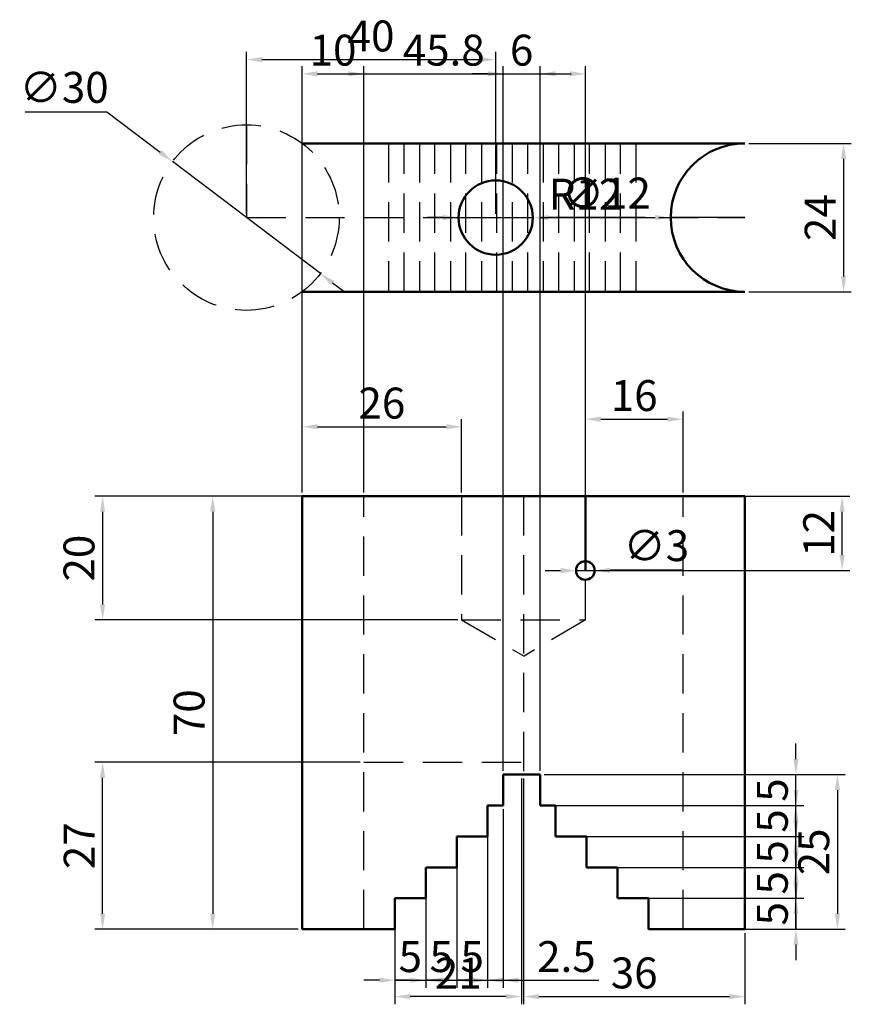
# Model space of a CAD drawing. Units: millimetres. Extents: x 1338 to 1892, y 1867 to 2306.
# Tile 1 of 3: x 1338 to 1473, y 1867 to 2026. Entities that reach past the tile are written whole.
import ezdxf

# ---------------------------------------------------------------- set-up
doc = ezdxf.new("R2010")
doc.units = ezdxf.units.MM
doc.linetypes.add('HIDDEN', pattern=[9.525, 6.35, -3.175])
for name, color, linetype, lineweight in [('M-DIMS', 2, 'Continuous', 25), ('M-HIDN', 4, 'HIDDEN', 25), ('M-OUTL', 7, 'Continuous', 50)]:
    doc.layers.add(name, color=color, linetype=linetype, lineweight=lineweight)
doc.styles.get("Standard").update_dxf_attribs({"font": 'arial.ttf'})
doc.dimstyles.new('ISO-25', dxfattribs={"dimtxt": 5, "dimasz": 2.5, "dimexe": 1.25, "dimexo": 0.625, "dimtad": 1, "dimtoh": 1, "dimdec": 0, "dimtxsty": 'Standard', "dimcen": 2.5, "dimadec": 0, "dimazin": 0, "dimtfac": 1, "dimtdec": 0, "dimtmove": 0, "dimatfit": 3, "dimfxl": 1, "dimarcsym": 0})

# ---------------------------------------------------------------- blocks, each defined once
blk = doc.blocks.new('*D16')
at = {"layer": 'Defpoints', "color": 0, "transparency": 16777216}
for p in [(1362.75, 2003.52), (1386.66, 1985.39)]:
    blk.add_point(p, dxfattribs=at)
at = {"layer": 'M-DIMS', "color": 0, "lineweight": -2, "transparency": 16777216}
for p, q in [((1338.95, 2011.54), (1352.16, 2011.54)), ((1352.16, 2011.54), (1360.76, 2005.03)), ((1386.66, 1985.39), (1362.75, 2003.52)), ((1388.65, 1983.88), (1390.65, 1982.37))]:
    blk.add_line(p, q, dxfattribs=at)
at = {"layer": 'M-DIMS', "color": 0, "transparency": 16777216}
for points in [[(1361.01, 2005.36), (1360.51, 2004.69), (1362.75, 2003.52)], [(1388.91, 1984.22), (1388.4, 1983.55), (1386.66, 1985.39)]]:
    blk.add_solid(points, dxfattribs=at)
at = {"layer": 'M-DIMS', "color": 0, "transparency": 16777216, "insert": (1345.24, 2014.86), "char_height": 5, "attachment_point": 5}
blk.add_mtext('∅30', dxfattribs=at)
blk = doc.blocks.new('*D17')
at = {"layer": 'Defpoints', "color": 0, "transparency": 16777216}
for p in [(1415.01, 2019.99), (1374.71, 1994.45), (1415.01, 1994.45)]:
    blk.add_point(p, dxfattribs=at)
at = {"layer": 'M-DIMS', "color": 0, "lineweight": -2, "transparency": 16777216}
for p, q in [((1374.71, 1995.08), (1374.71, 2021.24)), ((1415.01, 1995.08), (1415.01, 2021.24)), ((1377.21, 2019.99), (1412.51, 2019.99))]:
    blk.add_line(p, q, dxfattribs=at)
at = {"layer": 'M-DIMS', "color": 0, "transparency": 16777216}
for points in [[(1377.21, 2020.41), (1377.21, 2019.58), (1374.71, 2019.99)], [(1412.51, 2020.41), (1412.51, 2019.58), (1415.01, 2019.99)]]:
    blk.add_solid(points, dxfattribs=at)
at = {"layer": 'M-DIMS', "color": 0, "transparency": 16777216, "insert": (1394.86, 2023.17), "char_height": 5, "attachment_point": 5}
blk.add_mtext('40', dxfattribs=at)
blk = doc.blocks.new('*D18')
at = {"layer": 'Defpoints', "color": 0, "transparency": 16777216}
for p in [(1455.31, 2006.45), (1455.31, 1982.45), (1471.26, 1982.45)]:
    blk.add_point(p, dxfattribs=at)
at = {"layer": 'M-DIMS', "color": 0, "lineweight": -2, "transparency": 16777216}
for p, q in [((1455.93, 2006.45), (1472.51, 2006.45)), ((1471.26, 2003.95), (1471.26, 1984.95)), ((1455.93, 1982.45), (1472.51, 1982.45))]:
    blk.add_line(p, q, dxfattribs=at)
at = {"layer": 'M-DIMS', "color": 0, "transparency": 16777216}
for points in [[(1470.84, 2003.95), (1471.68, 2003.95), (1471.26, 2006.45)], [(1470.84, 1984.95), (1471.68, 1984.95), (1471.26, 1982.45)]]:
    blk.add_solid(points, dxfattribs=at)
at = {"layer": 'M-DIMS', "color": 0, "transparency": 16777216, "insert": (1468.13, 1994.45), "char_height": 5, "attachment_point": 5, "rotation": 90}
blk.add_mtext('24', dxfattribs=at)
blk = doc.blocks.new('*D19')
at = {"layer": 'Defpoints', "color": 0, "transparency": 16777216}
for p in [(1383.71, 1949.39), (1369.26, 1879.39), (1383.71, 1879.39)]:
    blk.add_point(p, dxfattribs=at)
at = {"layer": 'M-DIMS', "color": 0, "lineweight": -2, "transparency": 16777216}
for p, q in [((1383.08, 1949.39), (1368.01, 1949.39)), ((1369.26, 1946.89), (1369.26, 1881.89)), ((1383.08, 1879.39), (1368.01, 1879.39))]:
    blk.add_line(p, q, dxfattribs=at)
at = {"layer": 'M-DIMS', "color": 0, "transparency": 16777216}
for points in [[(1368.84, 1946.89), (1369.68, 1946.89), (1369.26, 1949.39)], [(1368.84, 1881.89), (1369.68, 1881.89), (1369.26, 1879.39)]]:
    blk.add_solid(points, dxfattribs=at)
at = {"layer": 'M-DIMS', "color": 0, "transparency": 16777216, "insert": (1366.08, 1914.39), "char_height": 5, "attachment_point": 5, "rotation": 90}
blk.add_mtext('70', dxfattribs=at)
blk = doc.blocks.new('*D20')
at = {"layer": 'Defpoints', "color": 0, "transparency": 16777216}
for p in [(1419.21, 1904.39), (1398.71, 1879.39), (1398.71, 1868.49)]:
    blk.add_point(p, dxfattribs=at)
at = {"layer": 'M-DIMS', "color": 0, "lineweight": -2, "transparency": 16777216}
for p, q in [((1419.21, 1903.77), (1419.21, 1867.24)), ((1398.71, 1878.77), (1398.71, 1867.24)), ((1416.71, 1868.49), (1401.21, 1868.49))]:
    blk.add_line(p, q, dxfattribs=at)
at = {"layer": 'M-DIMS', "color": 0, "transparency": 16777216}
for points in [[(1401.21, 1868.91), (1401.21, 1868.08), (1398.71, 1868.49)], [(1416.71, 1868.91), (1416.71, 1868.08), (1419.21, 1868.49)]]:
    blk.add_solid(points, dxfattribs=at)
at = {"layer": 'M-DIMS', "color": 0, "transparency": 16777216, "insert": (1408.96, 1871.63), "char_height": 5, "attachment_point": 5}
blk.add_mtext('21', dxfattribs=at)
blk = doc.blocks.new('*D21')
at = {"layer": 'Defpoints', "color": 0, "transparency": 16777216}
for p in [(1419.51, 1904.39), (1455.31, 1879.39), (1455.31, 1868.49)]:
    blk.add_point(p, dxfattribs=at)
at = {"layer": 'M-DIMS', "color": 0, "lineweight": -2, "transparency": 16777216}
for p, q in [((1419.51, 1903.77), (1419.51, 1867.24)), ((1455.31, 1878.77), (1455.31, 1867.24)), ((1422.01, 1868.49), (1452.81, 1868.49))]:
    blk.add_line(p, q, dxfattribs=at)
at = {"layer": 'M-DIMS', "color": 0, "transparency": 16777216}
for points in [[(1422.01, 1868.91), (1422.01, 1868.08), (1419.51, 1868.49)], [(1452.81, 1868.91), (1452.81, 1868.08), (1455.31, 1868.49)]]:
    blk.add_solid(points, dxfattribs=at)
at = {"layer": 'M-DIMS', "color": 0, "transparency": 16777216, "insert": (1437.41, 1871.67), "char_height": 5, "attachment_point": 5}
blk.add_mtext('36', dxfattribs=at)
blk = doc.blocks.new('*D22')
at = {"layer": 'Defpoints', "color": 0, "transparency": 16777216}
for p in [(1422.21, 1904.39), (1455.31, 1879.39), (1470.27, 1879.39)]:
    blk.add_point(p, dxfattribs=at)
at = {"layer": 'M-DIMS', "color": 0, "lineweight": -2, "transparency": 16777216}
for p, q in [((1422.83, 1904.39), (1471.52, 1904.39)), ((1470.27, 1901.89), (1470.27, 1881.89)), ((1455.93, 1879.39), (1471.52, 1879.39))]:
    blk.add_line(p, q, dxfattribs=at)
at = {"layer": 'M-DIMS', "color": 0, "transparency": 16777216}
for points in [[(1469.85, 1901.89), (1470.69, 1901.89), (1470.27, 1904.39)], [(1469.85, 1881.89), (1470.69, 1881.89), (1470.27, 1879.39)]]:
    blk.add_solid(points, dxfattribs=at)
at = {"layer": 'M-DIMS', "color": 0, "transparency": 16777216, "insert": (1467.09, 1891.89), "char_height": 5, "attachment_point": 5, "rotation": 90}
blk.add_mtext('25', dxfattribs=at)
blk = doc.blocks.new('*D23')
at = {"layer": 'Defpoints', "color": 0, "transparency": 16777216}
for p in [(1445.31, 1961.86), (1429.51, 1949.39), (1445.31, 1949.39)]:
    blk.add_point(p, dxfattribs=at)
at = {"layer": 'M-DIMS', "color": 0, "lineweight": -2, "transparency": 16777216}
for p, q in [((1429.51, 1950.02), (1429.51, 1963.11)), ((1445.31, 1950.02), (1445.31, 1963.11)), ((1432.01, 1961.86), (1442.81, 1961.86))]:
    blk.add_line(p, q, dxfattribs=at)
at = {"layer": 'M-DIMS', "color": 0, "transparency": 16777216}
for points in [[(1432.01, 1962.27), (1432.01, 1961.44), (1429.51, 1961.86)], [(1442.81, 1962.27), (1442.81, 1961.44), (1445.31, 1961.86)]]:
    blk.add_solid(points, dxfattribs=at)
at = {"layer": 'M-DIMS', "color": 0, "transparency": 16777216, "insert": (1437.41, 1965.03), "char_height": 5, "attachment_point": 5}
blk.add_mtext('16', dxfattribs=at)
blk = doc.blocks.new('*D24')
at = {"layer": 'Defpoints', "color": 0, "transparency": 16777216}
for p in [(1409.51, 1960.63), (1383.71, 1949.39), (1409.51, 1949.39)]:
    blk.add_point(p, dxfattribs=at)
at = {"layer": 'M-DIMS', "color": 0, "lineweight": -2, "transparency": 16777216}
for p, q in [((1383.71, 1950.02), (1383.71, 1961.88)), ((1409.51, 1950.02), (1409.51, 1961.88)), ((1386.21, 1960.63), (1407.01, 1960.63))]:
    blk.add_line(p, q, dxfattribs=at)
at = {"layer": 'M-DIMS', "color": 0, "transparency": 16777216}
for points in [[(1386.21, 1961.05), (1386.21, 1960.22), (1383.71, 1960.63)], [(1407.01, 1961.05), (1407.01, 1960.22), (1409.51, 1960.63)]]:
    blk.add_solid(points, dxfattribs=at)
at = {"layer": 'M-DIMS', "color": 0, "transparency": 16777216, "insert": (1396.61, 1963.81), "char_height": 5, "attachment_point": 5}
blk.add_mtext('26', dxfattribs=at)
blk = doc.blocks.new('*D25')
at = {"layer": 'Defpoints', "color": 0, "transparency": 16777216}
for p in [(1429.51, 1949.39), (1471.03, 1949.39), (1429.51, 1937.39)]:
    blk.add_point(p, dxfattribs=at)
at = {"layer": 'M-DIMS', "color": 0, "lineweight": -2, "transparency": 16777216}
for p, q in [((1430.13, 1949.39), (1472.28, 1949.39)), ((1471.03, 1939.89), (1471.03, 1946.89)), ((1430.13, 1937.39), (1472.28, 1937.39))]:
    blk.add_line(p, q, dxfattribs=at)
at = {"layer": 'M-DIMS', "color": 0, "transparency": 16777216}
for points in [[(1470.61, 1946.89), (1471.44, 1946.89), (1471.03, 1949.39)], [(1470.61, 1939.89), (1471.44, 1939.89), (1471.03, 1937.39)]]:
    blk.add_solid(points, dxfattribs=at)
at = {"layer": 'M-DIMS', "color": 0, "transparency": 16777216, "insert": (1467.89, 1943.39), "char_height": 5, "attachment_point": 5, "rotation": 90}
blk.add_mtext('12', dxfattribs=at)
blk = doc.blocks.new('*D58')
at = {"layer": 'Defpoints', "color": 0, "transparency": 16777216}
for p in [(1429.51, 2017.7), (1383.71, 1949.39), (1429.51, 1937.39)]:
    blk.add_point(p, dxfattribs=at)
at = {"layer": 'M-DIMS', "color": 0, "lineweight": -2, "transparency": 16777216}
for p, q in [((1383.71, 1950.02), (1383.71, 2018.95)), ((1429.51, 1938.02), (1429.51, 2018.95)), ((1386.21, 2017.7), (1427.01, 2017.7))]:
    blk.add_line(p, q, dxfattribs=at)
at = {"layer": 'M-DIMS', "color": 0, "transparency": 16777216}
for points in [[(1386.21, 2018.12), (1386.21, 2017.29), (1383.71, 2017.7)], [(1427.01, 2018.12), (1427.01, 2017.29), (1429.51, 2017.7)]]:
    blk.add_solid(points, dxfattribs=at)
at = {"layer": 'M-DIMS', "color": 0, "transparency": 16777216, "insert": (1406.61, 2020.88), "char_height": 5, "attachment_point": 5}
blk.add_mtext('45.8', dxfattribs=at)
blk = doc.blocks.new('*D59')
at = {"layer": 'Defpoints', "color": 0, "transparency": 16777216}
for p in [(1409.51, 1949.39), (1351.46, 1929.39), (1409.51, 1929.39)]:
    blk.add_point(p, dxfattribs=at)
at = {"layer": 'M-DIMS', "color": 0, "lineweight": -2, "transparency": 16777216}
for p, q in [((1408.88, 1949.39), (1350.21, 1949.39)), ((1351.46, 1946.89), (1351.46, 1931.89)), ((1408.88, 1929.39), (1350.21, 1929.39))]:
    blk.add_line(p, q, dxfattribs=at)
at = {"layer": 'M-DIMS', "color": 0, "transparency": 16777216}
for points in [[(1351.04, 1946.89), (1351.87, 1946.89), (1351.46, 1949.39)], [(1351.04, 1931.89), (1351.87, 1931.89), (1351.46, 1929.39)]]:
    blk.add_solid(points, dxfattribs=at)
at = {"layer": 'M-DIMS', "color": 0, "transparency": 16777216, "insert": (1348.28, 1939.39), "char_height": 5, "attachment_point": 5, "rotation": 90}
blk.add_mtext('20', dxfattribs=at)
blk = doc.blocks.new('*D60')
at = {"layer": 'Defpoints', "color": 0, "transparency": 16777216}
for p in [(1351.46, 1906.39), (1393.71, 1906.39), (1383.71, 1879.39)]:
    blk.add_point(p, dxfattribs=at)
at = {"layer": 'M-DIMS', "color": 0, "lineweight": -2, "transparency": 16777216}
for p, q in [((1393.08, 1906.39), (1350.21, 1906.39)), ((1351.46, 1881.89), (1351.46, 1903.89)), ((1383.08, 1879.39), (1350.21, 1879.39))]:
    blk.add_line(p, q, dxfattribs=at)
at = {"layer": 'M-DIMS', "color": 0, "transparency": 16777216}
for points in [[(1351.04, 1903.89), (1351.87, 1903.89), (1351.46, 1906.39)], [(1351.04, 1881.89), (1351.87, 1881.89), (1351.46, 1879.39)]]:
    blk.add_solid(points, dxfattribs=at)
at = {"layer": 'M-DIMS', "color": 0, "transparency": 16777216, "insert": (1348.32, 1892.89), "char_height": 5, "attachment_point": 5, "rotation": 90}
blk.add_mtext('27', dxfattribs=at)
blk = doc.blocks.new('*D61')
at = {"layer": 'Defpoints', "color": 0, "transparency": 16777216}
for p in [(1393.71, 2017.7), (1383.71, 1949.39), (1393.71, 1949.39)]:
    blk.add_point(p, dxfattribs=at)
at = {"layer": 'M-DIMS', "color": 0, "lineweight": -2, "transparency": 16777216}
for p, q in [((1383.71, 1950.02), (1383.71, 2018.95)), ((1393.71, 1950.02), (1393.71, 2018.95)), ((1386.21, 2017.7), (1391.21, 2017.7))]:
    blk.add_line(p, q, dxfattribs=at)
at = {"layer": 'M-DIMS', "color": 0, "transparency": 16777216}
for points in [[(1386.21, 2018.12), (1386.21, 2017.29), (1383.71, 2017.7)], [(1391.21, 2018.12), (1391.21, 2017.29), (1393.71, 2017.7)]]:
    blk.add_solid(points, dxfattribs=at)
at = {"layer": 'M-DIMS', "color": 0, "transparency": 16777216, "insert": (1388.71, 2020.88), "char_height": 5, "attachment_point": 5}
blk.add_mtext('10', dxfattribs=at)
blk = doc.blocks.new('*D62')
at = {"layer": 'Defpoints', "color": 0, "transparency": 16777216}
for p in [(1398.71, 1884.39), (1403.71, 1884.39), (1403.71, 1871.14)]:
    blk.add_point(p, dxfattribs=at)
at = {"layer": 'M-DIMS', "color": 0, "lineweight": -2, "transparency": 16777216}
for p, q in [((1398.71, 1883.77), (1398.71, 1869.89)), ((1403.71, 1883.77), (1403.71, 1869.89)), ((1396.21, 1871.14), (1393.71, 1871.14)), ((1398.71, 1871.14), (1403.71, 1871.14)), ((1406.21, 1871.14), (1408.71, 1871.14))]:
    blk.add_line(p, q, dxfattribs=at)
at = {"layer": 'M-DIMS', "color": 0, "transparency": 16777216}
for points in [[(1396.21, 1871.56), (1396.21, 1870.72), (1398.71, 1871.14)], [(1406.21, 1871.56), (1406.21, 1870.72), (1403.71, 1871.14)]]:
    blk.add_solid(points, dxfattribs=at)
at = {"layer": 'M-DIMS', "color": 0, "transparency": 16777216, "insert": (1401.21, 1874.31), "char_height": 5, "attachment_point": 5}
blk.add_mtext('5', dxfattribs=at)
blk = doc.blocks.new('*D63')
at = {"layer": 'Defpoints', "color": 0, "transparency": 16777216}
for p in [(1403.71, 1889.39), (1408.71, 1889.39), (1408.71, 1871.14)]:
    blk.add_point(p, dxfattribs=at)
at = {"layer": 'M-DIMS', "color": 0, "lineweight": -2, "transparency": 16777216}
for p, q in [((1403.71, 1888.77), (1403.71, 1869.89)), ((1408.71, 1888.77), (1408.71, 1869.89)), ((1401.21, 1871.14), (1398.71, 1871.14)), ((1403.71, 1871.14), (1408.71, 1871.14)), ((1411.21, 1871.14), (1413.71, 1871.14))]:
    blk.add_line(p, q, dxfattribs=at)
at = {"layer": 'M-DIMS', "color": 0, "transparency": 16777216}
for points in [[(1401.21, 1871.56), (1401.21, 1870.72), (1403.71, 1871.14)], [(1411.21, 1871.56), (1411.21, 1870.72), (1408.71, 1871.14)]]:
    blk.add_solid(points, dxfattribs=at)
at = {"layer": 'M-DIMS', "color": 0, "transparency": 16777216, "insert": (1406.21, 1874.31), "char_height": 5, "attachment_point": 5}
blk.add_mtext('5', dxfattribs=at)
blk = doc.blocks.new('*D64')
at = {"layer": 'Defpoints', "color": 0, "transparency": 16777216}
for p in [(1408.71, 1894.39), (1413.71, 1894.39), (1413.71, 1871.14)]:
    blk.add_point(p, dxfattribs=at)
at = {"layer": 'M-DIMS', "color": 0, "lineweight": -2, "transparency": 16777216}
for p, q in [((1408.71, 1893.77), (1408.71, 1869.89)), ((1413.71, 1893.77), (1413.71, 1869.89)), ((1406.21, 1871.14), (1403.71, 1871.14)), ((1408.71, 1871.14), (1413.71, 1871.14)), ((1416.21, 1871.14), (1418.71, 1871.14))]:
    blk.add_line(p, q, dxfattribs=at)
at = {"layer": 'M-DIMS', "color": 0, "transparency": 16777216}
for points in [[(1406.21, 1871.56), (1406.21, 1870.72), (1408.71, 1871.14)], [(1416.21, 1871.56), (1416.21, 1870.72), (1413.71, 1871.14)]]:
    blk.add_solid(points, dxfattribs=at)
at = {"layer": 'M-DIMS', "color": 0, "transparency": 16777216, "insert": (1411.21, 1874.31), "char_height": 5, "attachment_point": 5}
blk.add_mtext('5', dxfattribs=at)
blk = doc.blocks.new('*D65')
at = {"layer": 'Defpoints', "color": 0, "transparency": 16777216}
for p in [(1413.71, 1899.39), (1416.21, 1899.39), (1416.21, 1871.14)]:
    blk.add_point(p, dxfattribs=at)
at = {"layer": 'M-DIMS', "color": 0, "lineweight": -2, "transparency": 16777216}
for p, q in [((1413.71, 1898.77), (1413.71, 1869.89)), ((1416.21, 1898.77), (1416.21, 1869.89)), ((1411.21, 1871.14), (1408.71, 1871.14)), ((1413.71, 1871.14), (1416.21, 1871.14)), ((1418.71, 1871.14), (1431.68, 1871.14))]:
    blk.add_line(p, q, dxfattribs=at)
at = {"layer": 'M-DIMS', "color": 0, "transparency": 16777216}
for points in [[(1411.21, 1871.56), (1411.21, 1870.72), (1413.71, 1871.14)], [(1418.71, 1871.56), (1418.71, 1870.72), (1416.21, 1871.14)]]:
    blk.add_solid(points, dxfattribs=at)
at = {"layer": 'M-DIMS', "color": 0, "transparency": 16777216, "insert": (1426.45, 1874.32), "char_height": 5, "attachment_point": 5}
blk.add_mtext('2.5', dxfattribs=at)
blk = doc.blocks.new('*D66')
at = {"layer": 'Defpoints', "color": 0, "transparency": 16777216}
for p in [(1422.21, 2017.7), (1416.21, 1904.39), (1422.21, 1904.39)]:
    blk.add_point(p, dxfattribs=at)
at = {"layer": 'M-DIMS', "color": 0, "lineweight": -2, "transparency": 16777216}
for p, q in [((1416.21, 1905.02), (1416.21, 2018.95)), ((1422.21, 1905.02), (1422.21, 2018.95)), ((1413.71, 2017.7), (1411.21, 2017.7)), ((1416.21, 2017.7), (1422.21, 2017.7)), ((1424.71, 2017.7), (1427.21, 2017.7))]:
    blk.add_line(p, q, dxfattribs=at)
at = {"layer": 'M-DIMS', "color": 0, "transparency": 16777216}
for points in [[(1413.71, 2018.12), (1413.71, 2017.29), (1416.21, 2017.7)], [(1424.71, 2018.12), (1424.71, 2017.29), (1422.21, 2017.7)]]:
    blk.add_solid(points, dxfattribs=at)
at = {"layer": 'M-DIMS', "color": 0, "transparency": 16777216, "insert": (1419.21, 2020.88), "char_height": 5, "attachment_point": 5}
blk.add_mtext('6', dxfattribs=at)
blk = doc.blocks.new('*D67')
at = {"layer": 'Defpoints', "color": 0, "transparency": 16777216}
for p in [(1439.71, 1884.39), (1463.56, 1884.39), (1439.71, 1879.39)]:
    blk.add_point(p, dxfattribs=at)
at = {"layer": 'M-DIMS', "color": 0, "lineweight": -2, "transparency": 16777216}
for p, q in [((1463.56, 1886.89), (1463.56, 1889.39)), ((1440.33, 1884.39), (1464.81, 1884.39)), ((1463.56, 1879.39), (1463.56, 1884.39)), ((1440.33, 1879.39), (1464.81, 1879.39)), ((1463.56, 1876.89), (1463.56, 1874.39))]:
    blk.add_line(p, q, dxfattribs=at)
at = {"layer": 'M-DIMS', "color": 0, "transparency": 16777216}
for points in [[(1463.14, 1886.89), (1463.97, 1886.89), (1463.56, 1884.39)], [(1463.14, 1876.89), (1463.97, 1876.89), (1463.56, 1879.39)]]:
    blk.add_solid(points, dxfattribs=at)
at = {"layer": 'M-DIMS', "color": 0, "transparency": 16777216, "insert": (1460.39, 1881.89), "char_height": 5, "attachment_point": 5, "rotation": 90}
blk.add_mtext('5', dxfattribs=at)
blk = doc.blocks.new('*D68')
at = {"layer": 'Defpoints', "color": 0, "transparency": 16777216}
for p in [(1434.71, 1889.39), (1463.56, 1889.39), (1434.71, 1884.39)]:
    blk.add_point(p, dxfattribs=at)
at = {"layer": 'M-DIMS', "color": 0, "lineweight": -2, "transparency": 16777216}
for p, q in [((1463.56, 1891.89), (1463.56, 1894.39)), ((1435.33, 1889.39), (1464.81, 1889.39)), ((1463.56, 1884.39), (1463.56, 1889.39)), ((1435.33, 1884.39), (1464.81, 1884.39)), ((1463.56, 1881.89), (1463.56, 1879.39))]:
    blk.add_line(p, q, dxfattribs=at)
at = {"layer": 'M-DIMS', "color": 0, "transparency": 16777216}
for points in [[(1463.14, 1891.89), (1463.97, 1891.89), (1463.56, 1889.39)], [(1463.14, 1881.89), (1463.97, 1881.89), (1463.56, 1884.39)]]:
    blk.add_solid(points, dxfattribs=at)
at = {"layer": 'M-DIMS', "color": 0, "transparency": 16777216, "insert": (1460.39, 1886.89), "char_height": 5, "attachment_point": 5, "rotation": 90}
blk.add_mtext('5', dxfattribs=at)
blk = doc.blocks.new('*D69')
at = {"layer": 'Defpoints', "color": 0, "transparency": 16777216}
for p in [(1429.71, 1894.39), (1463.56, 1894.39), (1429.71, 1889.39)]:
    blk.add_point(p, dxfattribs=at)
at = {"layer": 'M-DIMS', "color": 0, "lineweight": -2, "transparency": 16777216}
for p, q in [((1463.56, 1896.89), (1463.56, 1899.39)), ((1430.33, 1894.39), (1464.81, 1894.39)), ((1463.56, 1889.39), (1463.56, 1894.39)), ((1430.33, 1889.39), (1464.81, 1889.39)), ((1463.56, 1886.89), (1463.56, 1884.39))]:
    blk.add_line(p, q, dxfattribs=at)
at = {"layer": 'M-DIMS', "color": 0, "transparency": 16777216}
for points in [[(1463.14, 1896.89), (1463.97, 1896.89), (1463.56, 1894.39)], [(1463.14, 1886.89), (1463.97, 1886.89), (1463.56, 1889.39)]]:
    blk.add_solid(points, dxfattribs=at)
at = {"layer": 'M-DIMS', "color": 0, "transparency": 16777216, "insert": (1460.39, 1891.89), "char_height": 5, "attachment_point": 5, "rotation": 90}
blk.add_mtext('5', dxfattribs=at)
blk = doc.blocks.new('*D70')
at = {"layer": 'Defpoints', "color": 0, "transparency": 16777216}
for p in [(1424.71, 1899.39), (1463.56, 1899.39), (1424.71, 1894.39)]:
    blk.add_point(p, dxfattribs=at)
at = {"layer": 'M-DIMS', "color": 0, "lineweight": -2, "transparency": 16777216}
for p, q in [((1463.56, 1901.89), (1463.56, 1904.39)), ((1425.33, 1899.39), (1464.81, 1899.39)), ((1463.56, 1894.39), (1463.56, 1899.39)), ((1425.33, 1894.39), (1464.81, 1894.39)), ((1463.56, 1891.89), (1463.56, 1889.39))]:
    blk.add_line(p, q, dxfattribs=at)
at = {"layer": 'M-DIMS', "color": 0, "transparency": 16777216}
for points in [[(1463.14, 1901.89), (1463.97, 1901.89), (1463.56, 1899.39)], [(1463.14, 1891.89), (1463.97, 1891.89), (1463.56, 1894.39)]]:
    blk.add_solid(points, dxfattribs=at)
at = {"layer": 'M-DIMS', "color": 0, "transparency": 16777216, "insert": (1460.39, 1896.89), "char_height": 5, "attachment_point": 5, "rotation": 90}
blk.add_mtext('5', dxfattribs=at)
blk = doc.blocks.new('*D71')
at = {"layer": 'Defpoints', "color": 0, "transparency": 16777216}
for p in [(1422.21, 1904.39), (1463.56, 1904.39), (1422.21, 1899.39)]:
    blk.add_point(p, dxfattribs=at)
at = {"layer": 'M-DIMS', "color": 0, "lineweight": -2, "transparency": 16777216}
for p, q in [((1463.56, 1906.89), (1463.56, 1909.39)), ((1422.83, 1904.39), (1464.81, 1904.39)), ((1463.56, 1899.39), (1463.56, 1904.39)), ((1422.83, 1899.39), (1464.81, 1899.39)), ((1463.56, 1896.89), (1463.56, 1894.39))]:
    blk.add_line(p, q, dxfattribs=at)
at = {"layer": 'M-DIMS', "color": 0, "transparency": 16777216}
for points in [[(1463.14, 1906.89), (1463.97, 1906.89), (1463.56, 1904.39)], [(1463.14, 1896.89), (1463.97, 1896.89), (1463.56, 1899.39)]]:
    blk.add_solid(points, dxfattribs=at)
at = {"layer": 'M-DIMS', "color": 0, "transparency": 16777216, "insert": (1460.39, 1901.89), "char_height": 5, "attachment_point": 5, "rotation": 90}
blk.add_mtext('5', dxfattribs=at)
blk = doc.blocks.new('*D76')
at = {"layer": 'Defpoints', "color": 0, "transparency": 16777216}
for p in [(1409.01, 1994.45), (1421.01, 1994.45)]:
    blk.add_point(p, dxfattribs=at)
at = {"layer": 'M-DIMS', "color": 0, "lineweight": -2, "transparency": 16777216}
for p, q in [((1406.51, 1994.45), (1404.01, 1994.45)), ((1409.01, 1994.45), (1421.01, 1994.45)), ((1426.01, 1994.46), (1423.51, 1994.46)), ((1439.18, 1994.46), (1426.01, 1994.46))]:
    blk.add_line(p, q, dxfattribs=at)
at = {"layer": 'M-DIMS', "color": 0, "transparency": 16777216}
for points in [[(1406.51, 1994.87), (1406.51, 1994.04), (1409.01, 1994.45)], [(1423.51, 1994.87), (1423.51, 1994.04), (1421.01, 1994.45)]]:
    blk.add_solid(points, dxfattribs=at)
at = {"layer": 'M-DIMS', "color": 0, "transparency": 16777216, "insert": (1432.91, 1997.77), "char_height": 5, "attachment_point": 5}
blk.add_mtext('∅12', dxfattribs=at)
blk = doc.blocks.new('*D77')
at = {"layer": 'Defpoints', "color": 0, "transparency": 16777216}
for p in [(1443.31, 1994.45), (1455.31, 1994.45)]:
    blk.add_point(p, dxfattribs=at)
at = {"layer": 'M-DIMS', "color": 0, "lineweight": -2, "transparency": 16777216}
for p, q in [((1423.59, 1994.46), (1436.11, 1994.46)), ((1436.11, 1994.46), (1440.81, 1994.45)), ((1455.31, 1994.45), (1443.31, 1994.45))]:
    blk.add_line(p, q, dxfattribs=at)
at = {"layer": 'M-DIMS', "color": 0, "transparency": 16777216}
blk.add_solid([(1440.81, 1994.87), (1440.81, 1994.04), (1443.31, 1994.45)], dxfattribs=at)
at = {"layer": 'M-DIMS', "color": 0, "transparency": 16777216, "insert": (1429.53, 1997.59), "char_height": 5, "attachment_point": 5}
blk.add_mtext('R12', dxfattribs=at)
blk = doc.blocks.new('*D78')
at = {"layer": 'Defpoints', "color": 0, "transparency": 16777216}
for p in [(1428.01, 1937.38), (1431.01, 1937.4)]:
    blk.add_point(p, dxfattribs=at)
at = {"layer": 'M-DIMS', "color": 0, "lineweight": -2, "transparency": 16777216}
for p, q in [((1425.51, 1937.36), (1423.01, 1937.34)), ((1428.01, 1937.38), (1431.01, 1937.4)), ((1436.01, 1937.44), (1433.51, 1937.42)), ((1445.35, 1937.44), (1436.01, 1937.44))]:
    blk.add_line(p, q, dxfattribs=at)
at = {"layer": 'M-DIMS', "color": 0, "transparency": 16777216}
for points in [[(1425.51, 1937.78), (1425.51, 1936.95), (1428.01, 1937.38)], [(1433.5, 1937.84), (1433.51, 1937), (1431.01, 1937.4)]]:
    blk.add_solid(points, dxfattribs=at)
at = {"layer": 'M-DIMS', "color": 0, "transparency": 16777216, "insert": (1440.99, 1940.76), "char_height": 5, "attachment_point": 5}
blk.add_mtext('∅3', dxfattribs=at)

msp = doc.modelspace()

# ---------------------------------------------------------------- linework, layer by layer
at = {"layer": 'M-HIDN'}
for p, q in [((1374.708, 2009.455), (1374.708, 1994.455)), ((1397.695, 2006.455), (1397.695, 1982.455)), ((1400.195, 1982.455), (1400.195, 2006.455)), ((1402.695, 2006.455), (1402.695, 1982.455)), ((1405.195, 1982.455), (1405.195, 2006.455)), ((1407.695, 2006.455), (1407.695, 1982.455)), ((1410.195, 1982.455), (1410.195, 2006.455)), ((1412.695, 2006.455), (1412.695, 1982.455)), ((1415.195, 1982.455), (1415.195, 2006.455)), ((1417.695, 2006.455), (1417.695, 1982.455)), ((1420.195, 1982.455), (1420.195, 2006.455)), ((1422.695, 2006.455), (1422.695, 1982.455)), ((1425.195, 1982.455), (1425.195, 2006.455)), ((1427.695, 2006.455), (1427.695, 1982.455)), ((1430.195, 1982.455), (1430.195, 2006.455)), ((1432.695, 2006.455), (1432.695, 1982.455)), ((1435.195, 1982.455), (1435.195, 2006.455)), ((1437.695, 2006.455), (1437.695, 1982.455)), ((1374.708, 1994.455), (1455.308, 1994.455)), ((1393.708, 1879.391), (1393.708, 1949.391)), ((1419.508, 1949.391), (1409.508, 1949.391)), ((1409.508, 1949.391), (1409.508, 1929.391)), ((1419.508, 1949.391), (1419.508, 1904.391)), ((1429.508, 1929.391), (1429.508, 1949.391)), ((1445.308, 1879.391), (1445.308, 1949.391)), ((1409.508, 1929.391), (1429.508, 1929.391)), ((1409.508, 1929.391), (1419.601, 1923.543)), ((1429.508, 1929.391), (1419.601, 1923.543)), ((1393.708, 1879.391), (1393.708, 1906.391)), ((1393.708, 1906.391), (1419.508, 1906.391))]:
    msp.add_line(p, q, dxfattribs=at)
msp.add_circle((1374.708, 1994.455), 15, dxfattribs=at)
at = {"layer": 'M-OUTL'}
for p, q in [((1455.308, 2006.455), (1383.708, 2006.455)), ((1455.308, 1982.455), (1383.708, 1982.455)), ((1383.708, 1949.391), (1455.308, 1949.391)), ((1383.708, 1949.391), (1383.708, 1879.391)), ((1429.508, 1949.391), (1429.508, 1937.391)), ((1455.308, 1949.391), (1455.308, 1879.391)), ((1416.208, 1899.391), (1416.208, 1904.391)), ((1416.208, 1904.391), (1422.208, 1904.391)), ((1422.208, 1904.391), (1422.208, 1899.391)), ((1413.708, 1894.391), (1413.708, 1899.391)), ((1413.708, 1899.391), (1416.208, 1899.391)), ((1422.208, 1899.391), (1424.708, 1899.391)), ((1424.708, 1899.391), (1424.708, 1894.391)), ((1408.708, 1889.391), (1408.708, 1894.391)), ((1408.708, 1894.391), (1413.708, 1894.391)), ((1424.708, 1894.391), (1429.708, 1894.391)), ((1429.708, 1894.391), (1429.708, 1889.391)), ((1403.708, 1884.391), (1403.708, 1889.391)), ((1403.708, 1889.391), (1408.708, 1889.391)), ((1429.708, 1889.391), (1434.708, 1889.391)), ((1434.708, 1889.391), (1434.708, 1884.391)), ((1398.708, 1879.391), (1398.708, 1884.391)), ((1398.708, 1884.391), (1403.708, 1884.391)), ((1434.708, 1884.391), (1439.708, 1884.391)), ((1439.708, 1884.391), (1439.708, 1879.391)), ((1383.708, 1879.391), (1393.708, 1879.391)), ((1393.708, 1879.391), (1398.708, 1879.391)), ((1439.708, 1879.391), (1445.308, 1879.391)), ((1455.308, 1879.391), (1445.308, 1879.391))]:
    msp.add_line(p, q, dxfattribs=at)
for centre, radius in [((1415.008, 1994.455), 6), ((1429.508, 1937.391), 1.5)]:
    msp.add_circle(centre, radius, dxfattribs=at)
msp.add_arc((1455.308, 1994.455), 12, 90, 270, dxfattribs=at)

# ---------------------------------------------------------------- dimensions: what is measured, and where the dimension line sits
at = {"layer": 'M-DIMS'}
for base, p1, p2, override, picture, middle in [((1415.008, 2019.993), (1374.708, 1994.455), (1415.008, 1994.455), {"dimclrd": 0, "dimclre": 0, "dimclrt": 0}, '*D17', (1394.858, 2023.171)), ((1429.508, 2017.705), (1383.708, 1949.391), (1429.508, 1937.391), {"dimdec": 1, "dimlfac": 1, "dimrnd": 0, "dimzin": 0, "dimdsep": 46, "dimlunit": 2}, '*D58', (1406.608, 2020.882)), ((1393.708, 2017.705), (1383.708, 1949.391), (1393.708, 1949.391), {"dimdec": 0, "dimlfac": 1, "dimrnd": 0, "dimzin": 0, "dimdsep": 46, "dimlunit": 2}, '*D61', (1388.708, 2020.882)), ((1422.208, 2017.705), (1416.208, 1904.391), (1422.208, 1904.391), {"dimdec": 0, "dimlfac": 1, "dimrnd": 0, "dimzin": 0, "dimdsep": 46, "dimlunit": 2}, '*D66', (1419.208, 2020.882)), ((1445.308, 1961.857), (1429.508, 1949.391), (1445.308, 1949.391), {"dimclrd": 0, "dimclre": 0, "dimclrt": 0}, '*D23', (1437.408, 1965.035)), ((1409.508, 1960.632), (1383.708, 1949.391), (1409.508, 1949.391), {"dimclrd": 0, "dimclre": 0, "dimclrt": 0}, '*D24', (1396.608, 1963.81)), ((1398.707980663, 1868.493183078), (1419.207980663, 1904.390716567), (1398.707980663, 1879.390716567), {"dimclrd": 0, "dimclre": 0, "dimclrt": 0}, '*D20', (1408.957980663, 1871.628415002)), ((1455.308, 1868.493), (1419.508, 1904.391), (1455.308, 1879.391), {"dimclrd": 0, "dimclre": 0, "dimclrt": 0}, '*D21', (1437.408, 1871.673)), ((1416.208, 1871.141), (1413.708, 1899.391), (1416.208, 1899.391), {"dimdec": 1, "dimlfac": 1, "dimrnd": 0, "dimzin": 0, "dimdsep": 46, "dimlunit": 2}, '*D65', (1426.446, 1874.319)), ((1413.708, 1871.141), (1408.708, 1894.391), (1413.708, 1894.391), {"dimdec": 0, "dimlfac": 1, "dimrnd": 0, "dimzin": 0, "dimdsep": 46, "dimlunit": 2}, '*D64', (1411.208, 1874.308)), ((1408.708, 1871.141), (1403.708, 1889.391), (1408.708, 1889.391), {"dimdec": 0, "dimlfac": 1, "dimrnd": 0, "dimzin": 0, "dimdsep": 46, "dimlunit": 2}, '*D63', (1406.208, 1874.308)), ((1403.708, 1871.141), (1398.708, 1884.391), (1403.708, 1884.391), {"dimdec": 0, "dimlfac": 1, "dimrnd": 0, "dimzin": 0, "dimdsep": 46, "dimlunit": 2}, '*D62', (1401.208, 1874.308))]:
    dim = msp.add_linear_dim(base=base, p1=p1, p2=p2, dimstyle='ISO-25', override=override, dxfattribs=at)
    dim.commit()
    dim.dimension.update_dxf_attribs({"geometry": picture, "text_midpoint": middle})
for p1, p2, override, picture, middle in [((1386.662, 1985.394), (1362.754, 2003.515), {"dimclrd": 0, "dimclre": 0, "dimclrt": 0}, '*D16', (1345.244, 2011.543)), ((1409.008, 1994.454), (1421.008, 1994.455), {"dimdec": 0, "dimlfac": 1, "dimrnd": 0, "dimzin": 0, "dimdsep": 46, "dimlunit": 2}, '*D76', (1426.008, 1994.455)), ((1428.008, 1937.38), (1431.008, 1937.401), {"dimdec": 0, "dimlfac": 1, "dimrnd": 0, "dimzin": 0, "dimdsep": 46, "dimlunit": 2}, '*D78', (1436.008, 1937.437))]:
    dim = msp.add_diameter_dim_2p(p1=p1, p2=p2, dimstyle='ISO-25', override=override, dxfattribs=at)
    dim.commit()
    dim.dimension.update_dxf_attribs({"geometry": picture, "text_midpoint": middle, "dimtype": 163})
for base, p1, p2, override, picture, middle in [((1471.261, 1982.455), (1455.308, 2006.455), (1455.308, 1982.455), {"dimclrd": 0, "dimclre": 0, "dimclrt": 0}, '*D18', (1468.126, 1994.455)), ((1351.458, 1929.391), (1409.508, 1949.391), (1409.508, 1929.391), {"dimdec": 0, "dimlfac": 1, "dimrnd": 0, "dimzin": 0, "dimdsep": 46, "dimlunit": 2}, '*D59', (1348.28, 1939.391)), ((1369.259, 1879.391), (1383.708, 1949.391), (1383.708, 1879.391), {"dimclrd": 0, "dimclre": 0, "dimclrt": 0}, '*D19', (1366.081, 1914.391)), ((1471.027, 1949.391), (1429.508, 1937.391), (1429.508, 1949.391), {"dimclrd": 0, "dimclre": 0, "dimclrt": 0}, '*D25', (1467.891, 1943.391)), ((1463.558, 1904.391), (1422.208, 1899.391), (1422.208, 1904.391), {"dimdec": 0, "dimlfac": 1, "dimrnd": 0, "dimzin": 0, "dimdsep": 46, "dimlunit": 2}, '*D71', (1460.39, 1901.891)), ((1351.458, 1906.391), (1383.708, 1879.391), (1393.708, 1906.391), {"dimdec": 0, "dimlfac": 1, "dimrnd": 0, "dimzin": 0, "dimdsep": 46, "dimlunit": 2}, '*D60', (1348.323, 1892.891)), ((1470.27, 1879.391), (1422.208, 1904.391), (1455.308, 1879.391), {"dimclrd": 0, "dimclre": 0, "dimclrt": 0}, '*D22', (1467.092, 1891.891)), ((1463.558, 1899.391), (1424.708, 1894.391), (1424.708, 1899.391), {"dimdec": 0, "dimlfac": 1, "dimrnd": 0, "dimzin": 0, "dimdsep": 46, "dimlunit": 2}, '*D70', (1460.39, 1896.891)), ((1463.558, 1894.391), (1429.708, 1889.391), (1429.708, 1894.391), {"dimdec": 0, "dimlfac": 1, "dimrnd": 0, "dimzin": 0, "dimdsep": 46, "dimlunit": 2}, '*D69', (1460.39, 1891.891)), ((1463.558, 1889.391), (1434.708, 1884.391), (1434.708, 1889.391), {"dimdec": 0, "dimlfac": 1, "dimrnd": 0, "dimzin": 0, "dimdsep": 46, "dimlunit": 2}, '*D68', (1460.39, 1886.891)), ((1463.558, 1884.391), (1439.708, 1879.391), (1439.708, 1884.391), {"dimdec": 0, "dimlfac": 1, "dimrnd": 0, "dimzin": 0, "dimdsep": 46, "dimlunit": 2}, '*D67', (1460.39, 1881.891))]:
    dim = msp.add_linear_dim(base=base, p1=p1, p2=p2, angle=90, dimstyle='ISO-25', override=override, dxfattribs=at)
    dim.commit()
    dim.dimension.update_dxf_attribs({"geometry": picture, "text_midpoint": middle})
dim = msp.add_radius_dim(center=(1455.308, 1994.455), mpoint=(1443.308, 1994.455), dimstyle='ISO-25', override={"dimdec": 0, "dimlfac": 1, "dimrnd": 0, "dimzin": 0, "dimdsep": 46, "dimlunit": 2}, dxfattribs=at)
dim.commit()
dim.dimension.update_dxf_attribs({"geometry": '*D77', "text_midpoint": (1436.108, 1994.455), "dimtype": 164})

doc.saveas('drawing.dxf')
